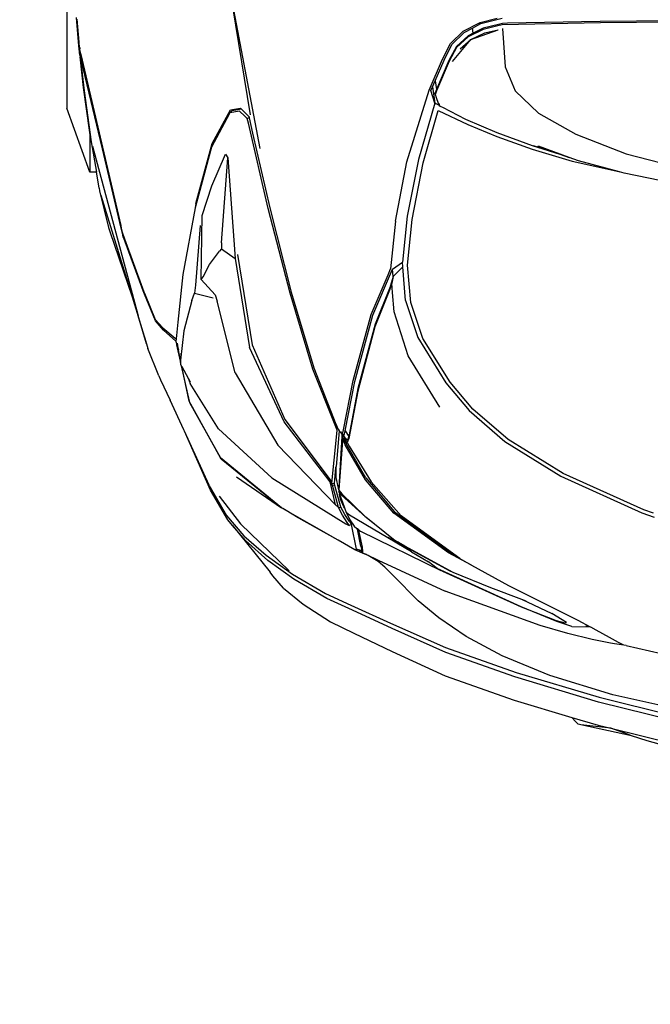
# Model space of a CAD drawing. Units: inches. Extents: x 22042254 to 25404563, y 17568978 to 17626777.
# Tile 21 of 45: x 22179809 to 22179830, y 17626194 to 17626227. Entities that reach past the tile are written whole.
import ezdxf

# ---------------------------------------------------------------- set-up
doc = ezdxf.new("R2010")
doc.units = ezdxf.units.IN
doc.header["$MEASUREMENT"] = 0
doc.layers.add('A-ANNO-DIMS', color=2, linetype='Continuous', lineweight=18)
doc.layers.add('A-SITE-VEHI', color=8, linetype='Continuous', lineweight=18)
doc.layers.add('Edges', color=250, linetype='Continuous')
doc.styles.get("Standard").update_dxf_attribs({"font": 'arial.ttf'})
doc.dimstyles.get("Standard").update_dxf_attribs({"dimtxt": 8, "dimasz": 0.18, "dimexe": 0.18, "dimexo": 0.0625, "dimgap": 0.09, "dimtad": 0, "dimtih": 1, "dimtoh": 1, "dimzin": 0, "dimdsep": 46, "dimlunit": 3, "dimtxsty": 'Standard', "dimcen": 0.09, "dimadec": 0, "dimazin": 0, "dimtfac": 1, "dimtofl": 0, "dimtmove": 0, "dimatfit": 3, "dimfxl": 1, "dimtolj": 1, "dimtzin": 0, "dimarcsym": 0})

# ---------------------------------------------------------------- blocks, each defined once
blk = doc.blocks.new('Nissan Qashqai pl')
at = {"layer": 'Edges'}
for p, q in [((11.05947, 11.55994), (11.06074, 11.45082)), ((11.06059, 11.56009), (11.06182, 11.4509)), ((11.6016, 11.52761), (11.58664, 11.46068)), ((11.58843, 11.44985), (11.60765, 11.5276)), ((11.61178, 11.52762), (11.59225, 11.44945)), ((11.61272, 11.45895), (11.62966, 11.52759)), ((11.16395, 11.47112), (11.17758, 11.52307)), ((11.18773, 11.51111), (11.17906, 11.46956)), ((11.54814, 11.47101), (11.55707, 11.51104)), ((11.62771, 11.50627), (11.62241, 11.48743)), ((11.44474, 11.49242), (11.44218, 11.48476)), ((11.44453, 11.48334), (11.44778, 11.49299)), ((11.44218, 11.48476), (11.41383, 11.42186)), ((11.41588, 11.41997), (11.44453, 11.48334)), ((11.62241, 11.48743), (11.61848, 11.47528)), ((11.61848, 11.47528), (11.61008, 11.43562)), ((11.61848, 11.47528), (11.61742, 11.47198)), ((11.14869, 11.43161), (11.16395, 11.47112)), ((11.17808, 11.46592), (11.1694, 11.43374)), ((11.17797, 11.4652), (11.17808, 11.46592)), ((11.17906, 11.46956), (11.17808, 11.46592)), ((11.54554, 11.46484), (11.54721, 11.46841)), ((11.54814, 11.47101), (11.54666, 11.46197)), ((11.61742, 11.47198), (11.61272, 11.45895)), ((11.1699, 11.42889), (11.17797, 11.4652)), ((11.53572, 11.44731), (11.54162, 11.45783)), ((11.54162, 11.45783), (11.54554, 11.46484)), ((11.54611, 11.45874), (11.54336, 11.44449)), ((11.54666, 11.46197), (11.54611, 11.45874)), ((11.58664, 11.46068), (11.57152, 11.41151)), ((11.61272, 11.45895), (11.61008, 11.43562)), ((11.61028, 11.44915), (11.61272, 11.45895)), ((11.06074, 11.45082), (11.06214, 11.37845)), ((11.06182, 11.4509), (11.06324, 11.37414)), ((11.52833, 11.43321), (11.53335, 11.4428)), ((11.53261, 11.43965), (11.5333, 11.44225)), ((11.53313, 11.42848), (11.53354, 11.44315)), ((11.5333, 11.44225), (11.53335, 11.4428)), ((11.53335, 11.4428), (11.53354, 11.44315)), ((11.53354, 11.44315), (11.53572, 11.44731)), ((11.54336, 11.44449), (11.53855, 11.42543)), ((11.56912, 11.38501), (11.58843, 11.44985)), ((11.59225, 11.44945), (11.57263, 11.38419)), ((11.60419, 11.42861), (11.61028, 11.44915)), ((11.61008, 11.43562), (11.60938, 11.43347)), ((11.1323, 11.40268), (11.14869, 11.43161)), ((11.16047, 11.39766), (11.1699, 11.42889)), ((11.1694, 11.43374), (11.1668, 11.42651)), ((11.5202, 11.41712), (11.52833, 11.43321)), ((11.53313, 11.42848), (11.52922, 11.417)), ((11.59084, 11.38361), (11.60419, 11.42861)), ((11.60772, 11.43162), (11.60419, 11.42861)), ((11.60938, 11.43347), (11.60772, 11.43162)), ((11.15764, 11.39828), (11.16426, 11.41918)), ((11.15766, 11.39771), (11.16426, 11.41918)), ((11.1668, 11.42651), (11.1582, 11.40259)), ((11.16426, 11.41918), (11.15826, 11.40186)), ((11.16426, 11.41918), (11.1668, 11.42651)), ((11.41383, 11.42186), (11.38718, 11.37878)), ((11.38877, 11.37638), (11.41588, 11.41997)), ((11.53009, 11.42439), (11.52299, 11.41307)), ((11.52855, 11.41625), (11.53022, 11.42324)), ((11.53022, 11.42324), (11.53009, 11.42439)), ((11.53855, 11.42543), (11.53253, 11.4038)), ((11.50131, 11.37908), (11.5202, 11.41712)), ((11.5118, 11.38938), (11.52299, 11.41307)), ((11.52922, 11.417), (11.51787, 11.38901)), ((11.51787, 11.38901), (11.52855, 11.41625)), ((11.57152, 11.41151), (11.55624, 11.37411)), ((11.53253, 11.4038), (11.50574, 11.32965)), ((11.11477, 11.38434), (11.1323, 11.40268)), ((11.14751, 11.37001), (11.15766, 11.39771)), ((11.15051, 11.36998), (11.16047, 11.39766)), ((11.51787, 11.38901), (11.48801, 11.32337)), ((11.49005, 11.3275), (11.51787, 11.38901)), ((11.50277, 11.36495), (11.5118, 11.38938)), ((11.5118, 11.38938), (11.51304, 11.39274)), ((11.09618, 11.37663), (11.11477, 11.38434)), ((11.54963, 11.33002), (11.56912, 11.38501)), ((11.57263, 11.38419), (11.5535, 11.33028)), ((11.57164, 11.32969), (11.59084, 11.38361)), ((11.06236, 11.3576), (11.05822, 11.37418)), ((11.06214, 11.37845), (11.06222, 11.37449)), ((11.06222, 11.37449), (11.06303, 11.37135)), ((11.06324, 11.37414), (11.06408, 11.37085)), ((11.06624, 11.37435), (11.09618, 11.37663)), ((11.38718, 11.37878), (11.3635, 11.35125)), ((11.36451, 11.34835), (11.38877, 11.37638)), ((11.48518, 11.35017), (11.50131, 11.37908)), ((11.55624, 11.37411), (11.54097, 11.34593)), ((11.06139, 11.35691), (11.05807, 11.37037)), ((11.06303, 11.37135), (11.06594, 11.3594)), ((11.06408, 11.37085), (11.06692, 11.35921)), ((11.06961, 11.36056), (11.0671, 11.37109)), ((11.07472, 11.34981), (11.0671, 11.37109)), ((11.13692, 11.34555), (11.14751, 11.37001)), ((11.14123, 11.34726), (11.15051, 11.36998)), ((11.06594, 11.3594), (11.06978, 11.35164)), ((11.06692, 11.35921), (11.0727, 11.34754)), ((11.07472, 11.34981), (11.06961, 11.36056)), ((11.49086, 11.33567), (11.50277, 11.36495)), ((11.06818, 11.34377), (11.06139, 11.35691)), ((11.06584, 11.35092), (11.06236, 11.3576)), ((11.06978, 11.35164), (11.06584, 11.35092)), ((11.06918, 11.34452), (11.06584, 11.35092)), ((11.06978, 11.35164), (11.07183, 11.3475)), ((11.3635, 11.35125), (11.34251, 11.3336)), ((11.48518, 11.35017), (11.4758, 11.33232)), ((11.48012, 11.34111), (11.48518, 11.35017)), ((11.07787, 11.3339), (11.06818, 11.34377)), ((11.07866, 11.33492), (11.06918, 11.34452)), ((11.07183, 11.3475), (11.08018, 11.33842)), ((11.0727, 11.34754), (11.0809, 11.33858)), ((11.08206, 11.34125), (11.07472, 11.34981)), ((11.092, 11.33548), (11.07472, 11.34981)), ((11.12767, 11.32749), (11.13692, 11.34555)), ((11.13017, 11.32416), (11.14123, 11.34726)), ((11.34283, 11.33026), (11.36451, 11.34835)), ((11.54097, 11.34593), (11.52646, 11.32473)), ((11.09081, 11.32882), (11.07866, 11.33492)), ((11.08018, 11.33842), (11.09121, 11.33249)), ((11.0809, 11.33858), (11.09174, 11.33271)), ((11.48005, 11.341), (11.44669, 11.29536)), ((11.47038, 11.29841), (11.49086, 11.33567)), ((11.47876, 11.33901), (11.47454, 11.33252)), ((11.47876, 11.33901), (11.48005, 11.341)), ((11.48005, 11.341), (11.48012, 11.34111)), ((11.48966, 11.33337), (11.49086, 11.33567)), ((11.09022, 11.32753), (11.07787, 11.3339)), ((11.11439, 11.31711), (11.09022, 11.32753)), ((11.10704, 11.32181), (11.09081, 11.32882)), ((11.09121, 11.33249), (11.1138, 11.3229)), ((11.09174, 11.33271), (11.11486, 11.323)), ((11.12645, 11.32495), (11.12767, 11.32749)), ((11.30757, 11.30833), (11.34283, 11.33026)), ((11.34251, 11.3336), (11.3082, 11.31215)), ((11.44331, 11.28988), (11.47454, 11.33252)), ((11.4758, 11.33232), (11.44474, 11.28965)), ((11.46332, 11.28473), (11.48966, 11.33337)), ((11.47038, 11.29841), (11.48966, 11.33337)), ((11.48133, 11.27727), (11.50574, 11.32965)), ((11.48983, 11.32694), (11.48954, 11.32636)), ((11.48983, 11.32694), (11.49005, 11.3275)), ((11.53062, 11.28691), (11.54963, 11.33002)), ((11.5535, 11.33028), (11.53487, 11.28826)), ((11.55274, 11.28821), (11.57164, 11.32969)), ((11.10704, 11.32181), (11.1138, 11.3229)), ((11.11164, 11.31982), (11.10704, 11.32181)), ((11.11164, 11.31982), (11.1244, 11.32146)), ((11.11467, 11.31851), (11.11164, 11.31982)), ((11.1138, 11.3229), (11.11393, 11.32284)), ((11.11393, 11.32284), (11.1164, 11.32172)), ((11.1244, 11.32146), (11.11467, 11.31851)), ((11.11486, 11.323), (11.1172, 11.32196)), ((11.1164, 11.32172), (11.1172, 11.32196)), ((11.11744, 11.32189), (11.1164, 11.32172)), ((11.1172, 11.32196), (11.11744, 11.32189)), ((11.11744, 11.32189), (11.11997, 11.32267)), ((11.11997, 11.32267), (11.12459, 11.32429)), ((11.12604, 11.32481), (11.1244, 11.32146)), ((11.1244, 11.32146), (11.12591, 11.32476)), ((11.1244, 11.32146), (11.16836, 11.30873)), ((11.12459, 11.32429), (11.12591, 11.32476)), ((11.12466, 11.32442), (11.12595, 11.32486)), ((11.12478, 11.32467), (11.12595, 11.32486)), ((11.12595, 11.32486), (11.1251, 11.3253)), ((11.12591, 11.32476), (11.12595, 11.32486)), ((11.12591, 11.32476), (11.12604, 11.32481)), ((11.12595, 11.32486), (11.12626, 11.32554)), ((11.12595, 11.32486), (11.12607, 11.32488)), ((11.12604, 11.32481), (11.12645, 11.32495)), ((11.12607, 11.32488), (11.12604, 11.32481)), ((11.12631, 11.32537), (11.12607, 11.32488)), ((11.12607, 11.32488), (11.12645, 11.32495)), ((11.17121, 11.31245), (11.13017, 11.32416)), ((11.36192, 11.32544), (11.32179, 11.30083)), ((11.45883, 11.26345), (11.48954, 11.32636)), ((11.48801, 11.32337), (11.48281, 11.31653)), ((11.52646, 11.32473), (11.51313, 11.30854)), ((11.17021, 11.29978), (11.11439, 11.31711)), ((11.21523, 11.3038), (11.17121, 11.31245)), ((11.3082, 11.31215), (11.28005, 11.30276)), ((11.47499, 11.30324), (11.48281, 11.31653)), ((11.16836, 11.30873), (11.21271, 11.29983)), ((11.2509, 11.3003), (11.21523, 11.3038)), ((11.27848, 11.29865), (11.30757, 11.30833)), ((11.51313, 11.30854), (11.49329, 11.28912)), ((11.21656, 11.2908), (11.17021, 11.29978)), ((11.21271, 11.29983), (11.24875, 11.29618)), ((11.25238, 11.29648), (11.24875, 11.29618)), ((11.2541, 11.28846), (11.24875, 11.29618)), ((11.28005, 11.30276), (11.2509, 11.3003)), ((11.27848, 11.29865), (11.25238, 11.29648)), ((11.25238, 11.29648), (11.25993, 11.28891)), ((11.32179, 11.30083), (11.28736, 11.28974)), ((11.47499, 11.30324), (11.4462, 11.25482)), ((11.46746, 11.29312), (11.47026, 11.29821)), ((11.47026, 11.29821), (11.47038, 11.29841)), ((11.21656, 11.2908), (11.25377, 11.28706)), ((11.25993, 11.28891), (11.2541, 11.28846)), ((11.29, 11.2731), (11.2541, 11.28846)), ((11.25993, 11.28891), (11.25999, 11.28889)), ((11.25999, 11.28889), (11.26503, 11.28789)), ((11.25999, 11.28889), (11.26771, 11.28668)), ((11.27242, 11.28847), (11.26503, 11.28789)), ((11.28736, 11.28974), (11.27242, 11.28847)), ((11.41708, 11.26758), (11.44331, 11.28988)), ((11.44474, 11.28965), (11.41866, 11.26734)), ((11.42028, 11.27173), (11.44669, 11.29536)), ((11.44691, 11.26684), (11.46587, 11.29022)), ((11.46538, 11.28932), (11.44788, 11.2676)), ((11.46538, 11.28932), (11.46587, 11.29022)), ((11.46587, 11.29022), (11.46737, 11.29293)), ((11.46746, 11.29312), (11.46737, 11.29293)), ((11.49329, 11.28912), (11.48692, 11.28262)), ((11.25857, 11.28503), (11.25377, 11.28706)), ((11.28951, 11.27177), (11.25857, 11.28503)), ((11.26503, 11.28789), (11.27055, 11.28622)), ((11.26771, 11.28668), (11.26785, 11.28663)), ((11.26785, 11.28663), (11.29721, 11.27493)), ((11.27055, 11.28622), (11.29928, 11.27468)), ((11.48692, 11.28262), (11.48256, 11.27724)), ((11.51652, 11.25601), (11.53062, 11.28691)), ((11.53487, 11.28826), (11.52058, 11.25724)), ((11.53843, 11.2583), (11.55274, 11.28821)), ((11.34188, 11.25916), (11.29, 11.2731)), ((11.29721, 11.27493), (11.34742, 11.26142)), ((11.29928, 11.27468), (11.34932, 11.2614)), ((11.47707, 11.26812), (11.48133, 11.27727)), ((11.48256, 11.27724), (11.47783, 11.26953)), ((11.48133, 11.27727), (11.48217, 11.27864)), ((11.3411, 11.25789), (11.28951, 11.27177)), ((11.41708, 11.26758), (11.38507, 11.24911)), ((11.41866, 11.26734), (11.3914, 11.25156)), ((11.39234, 11.25471), (11.42028, 11.27173)), ((11.42958, 11.2488), (11.44691, 11.26684)), ((11.44788, 11.2676), (11.43028, 11.24852)), ((11.47783, 11.26953), (11.47588, 11.26517)), ((11.47707, 11.26812), (11.47588, 11.26517)), ((11.37955, 11.25028), (11.3411, 11.25789)), ((11.38043, 11.25154), (11.34188, 11.25916)), ((11.34742, 11.26142), (11.38475, 11.2543)), ((11.34932, 11.2614), (11.38634, 11.25437)), ((11.44984, 11.25529), (11.45491, 11.25868)), ((11.47278, 11.2604), (11.45351, 11.25651)), ((11.45491, 11.25868), (11.45678, 11.26054)), ((11.4564, 11.26086), (11.45669, 11.26088)), ((11.45652, 11.26104), (11.45688, 11.26111)), ((11.45678, 11.26054), (11.45714, 11.2609)), ((11.45714, 11.2609), (11.45732, 11.2612)), ((11.45729, 11.26188), (11.45734, 11.2619)), ((11.47041, 11.26385), (11.45732, 11.2612)), ((11.45732, 11.2612), (11.45781, 11.262)), ((11.45736, 11.26195), (11.45734, 11.2619)), ((11.45736, 11.26195), (11.45755, 11.26195)), ((11.45781, 11.262), (11.45883, 11.26345)), ((11.45781, 11.262), (11.46047, 11.26254)), ((11.46047, 11.26254), (11.46049, 11.26254)), ((11.46049, 11.26254), (11.47129, 11.26473)), ((11.47322, 11.2592), (11.46579, 11.24614)), ((11.47041, 11.26385), (11.47423, 11.26446)), ((11.47129, 11.26473), (11.47442, 11.26498)), ((11.47269, 11.26007), (11.47281, 11.2603)), ((11.47463, 11.26457), (11.47278, 11.2604)), ((11.47423, 11.26446), (11.47278, 11.2604)), ((11.47278, 11.2604), (11.47281, 11.2603)), ((11.47281, 11.2603), (11.47317, 11.26096)), ((11.47281, 11.2603), (11.47322, 11.2592)), ((11.47585, 11.26509), (11.47322, 11.2592)), ((11.47423, 11.26446), (11.47445, 11.26449)), ((11.47442, 11.26498), (11.47433, 11.26475)), ((11.47442, 11.26498), (11.47446, 11.26498)), ((11.47445, 11.26477), (11.47446, 11.26498)), ((11.47463, 11.26457), (11.47445, 11.26449)), ((11.47446, 11.26498), (11.47482, 11.26501)), ((11.47585, 11.26509), (11.47463, 11.26457)), ((11.47482, 11.26501), (11.47475, 11.26484)), ((11.47482, 11.26501), (11.47585, 11.26509)), ((11.47588, 11.26517), (11.47585, 11.26509)), ((11.52949, 11.24004), (11.53843, 11.2583)), ((11.38338, 11.24949), (11.37955, 11.25028)), ((11.38043, 11.25154), (11.38475, 11.2543)), ((11.38408, 11.25081), (11.38043, 11.25154)), ((11.38295, 11.24897), (11.38801, 11.25321)), ((11.38408, 11.25081), (11.38338, 11.24949)), ((11.38475, 11.2543), (11.38801, 11.25321)), ((11.38823, 11.2519), (11.38491, 11.2491)), ((11.38811, 11.25194), (11.3861, 11.25078)), ((11.38634, 11.25437), (11.38953, 11.25299)), ((11.3914, 11.25156), (11.3867, 11.24922)), ((11.38862, 11.25223), (11.38822, 11.252)), ((11.38862, 11.25223), (11.38823, 11.2519)), ((11.39063, 11.25338), (11.38862, 11.25223)), ((11.38953, 11.25299), (11.38862, 11.25223)), ((11.38953, 11.25299), (11.39234, 11.25471)), ((11.41698, 11.19425), (11.45295, 11.25195)), ((11.4397, 11.25049), (11.43368, 11.248)), ((11.43609, 11.24937), (11.44061, 11.25095)), ((11.44061, 11.25095), (11.4397, 11.25049)), ((11.44573, 11.25131), (11.43996, 11.24823)), ((11.44061, 11.25095), (11.44418, 11.2522)), ((11.44418, 11.2522), (11.44968, 11.25519)), ((11.4462, 11.25482), (11.44418, 11.2522)), ((11.45121, 11.25489), (11.44573, 11.25131)), ((11.45199, 11.25317), (11.44624, 11.24948)), ((11.44968, 11.25519), (11.44984, 11.25529)), ((11.44984, 11.25529), (11.45351, 11.25651)), ((11.45121, 11.25489), (11.45351, 11.25651)), ((11.45386, 11.25448), (11.45199, 11.25317)), ((11.45295, 11.25195), (11.45421, 11.25473)), ((11.45316, 11.25595), (11.45351, 11.25651)), ((11.45351, 11.25651), (11.45421, 11.25473)), ((11.45421, 11.25473), (11.45386, 11.25448)), ((11.47197, 11.25711), (11.47177, 11.25676)), ((11.50736, 11.23616), (11.51652, 11.25601)), ((11.52058, 11.25724), (11.51126, 11.23721)), ((11.33108, 11.22699), (11.37506, 11.24429)), ((11.37475, 11.24309), (11.33228, 11.22637)), ((11.38, 11.24532), (11.37475, 11.24309)), ((11.37506, 11.24429), (11.37524, 11.24436)), ((11.37506, 11.24429), (11.37621, 11.24429)), ((11.37922, 11.24593), (11.37524, 11.24436)), ((11.3763, 11.24436), (11.37524, 11.24436)), ((11.37922, 11.24593), (11.38041, 11.24692)), ((11.37933, 11.24631), (11.37922, 11.24593)), ((11.38533, 11.24487), (11.38, 11.24532)), ((11.38041, 11.24692), (11.38275, 11.24887)), ((11.38041, 11.24692), (11.40818, 11.24436)), ((11.38129, 11.24847), (11.38167, 11.2488)), ((11.38275, 11.24887), (11.38338, 11.24949)), ((11.38446, 11.24984), (11.38295, 11.24897)), ((11.38295, 11.24897), (11.38491, 11.2491)), ((11.38295, 11.24897), (11.38461, 11.24885)), ((11.38461, 11.24885), (11.38464, 11.24887)), ((11.38461, 11.24885), (11.38934, 11.2486)), ((11.38464, 11.24887), (11.38501, 11.24911)), ((11.38491, 11.2491), (11.38464, 11.24887)), ((11.38501, 11.24911), (11.38507, 11.24911)), ((11.38507, 11.24911), (11.3867, 11.24922)), ((11.42115, 11.24117), (11.38533, 11.24487)), ((11.3867, 11.24922), (11.3915, 11.24906)), ((11.38934, 11.2486), (11.42481, 11.24653)), ((11.3915, 11.24906), (11.42659, 11.2465)), ((11.3915, 11.19885), (11.4381, 11.24397)), ((11.41644, 11.24436), (11.40818, 11.24436)), ((11.40898, 11.24429), (11.40818, 11.24436)), ((11.40898, 11.24429), (11.4163, 11.24429)), ((11.4152, 11.24371), (11.40898, 11.24429)), ((11.4163, 11.24429), (11.4152, 11.24371)), ((11.42154, 11.24313), (11.4152, 11.24371)), ((11.41644, 11.24436), (11.4163, 11.24429)), ((11.41686, 11.24458), (11.41644, 11.24436)), ((11.4252, 11.2462), (11.41686, 11.24458)), ((11.42115, 11.24117), (11.42154, 11.24313)), ((11.42296, 11.24352), (11.42154, 11.24313)), ((11.43154, 11.24397), (11.42287, 11.24164)), ((11.42296, 11.24352), (11.42287, 11.24164)), ((11.43996, 11.24823), (11.42296, 11.24352)), ((11.42481, 11.24653), (11.42659, 11.2465)), ((11.42659, 11.2465), (11.4252, 11.2462)), ((11.42659, 11.2465), (11.42684, 11.24649)), ((11.42684, 11.24649), (11.42958, 11.2488)), ((11.42684, 11.24649), (11.42784, 11.24647)), ((11.43028, 11.24852), (11.42784, 11.24647)), ((11.42784, 11.24647), (11.42996, 11.24721)), ((11.4381, 11.24397), (11.42915, 11.24177)), ((11.42996, 11.24721), (11.43609, 11.24937)), ((11.43368, 11.248), (11.42996, 11.24721)), ((11.44027, 11.24637), (11.43154, 11.24397)), ((11.4381, 11.24397), (11.44027, 11.24637)), ((11.44027, 11.24637), (11.43996, 11.24823)), ((11.44624, 11.24948), (11.44027, 11.24637)), ((11.44114, 11.20281), (11.46562, 11.24583)), ((11.44697, 11.21272), (11.46562, 11.24583)), ((11.46562, 11.24583), (11.46579, 11.24614)), ((11.3715, 11.20434), (11.41772, 11.23895)), ((11.42033, 11.23975), (11.37334, 11.20375)), ((11.41772, 11.23895), (11.41931, 11.23998)), ((11.41915, 11.23969), (11.4194, 11.23996)), ((11.41931, 11.23998), (11.4196, 11.24017)), ((11.4194, 11.23996), (11.41931, 11.23998)), ((11.4194, 11.23996), (11.4196, 11.24017)), ((11.41958, 11.23992), (11.4194, 11.23996)), ((11.4196, 11.24017), (11.42014, 11.24052)), ((11.41984, 11.24006), (11.42014, 11.24052)), ((11.42014, 11.24052), (11.42115, 11.24117)), ((11.42915, 11.24177), (11.42033, 11.23975)), ((11.42287, 11.24164), (11.42033, 11.23975)), ((11.42178, 11.24134), (11.42115, 11.24117)), ((11.42287, 11.24164), (11.42178, 11.24134)), ((11.42216, 11.24127), (11.42178, 11.24134)), ((11.49236, 11.21027), (11.50736, 11.23616)), ((11.51126, 11.23721), (11.49628, 11.21137)), ((11.51576, 11.21859), (11.52949, 11.24004)), ((11.27199, 11.20923), (11.33108, 11.22699)), ((11.33228, 11.22637), (11.27276, 11.20843)), ((11.44697, 11.21272), (11.44114, 11.20281)), ((11.50327, 11.20341), (11.51576, 11.21859)), ((11.20627, 11.19262), (11.27199, 11.20923)), ((11.27276, 11.20843), (11.20665, 11.19145)), ((11.31316, 11.17892), (11.3715, 11.20434)), ((11.45306, 11.16974), (11.48975, 11.20767)), ((11.47745, 11.18983), (11.49236, 11.21027)), ((11.49628, 11.21137), (11.48154, 11.19102)), ((11.37334, 11.20375), (11.31527, 11.17691)), ((11.33497, 11.16556), (11.3915, 11.19885)), ((11.44046, 11.20182), (11.40144, 11.15414)), ((11.40216, 11.15476), (11.44046, 11.20182)), ((11.41633, 11.16662), (11.44046, 11.20182)), ((11.44081, 11.20225), (11.44046, 11.20182)), ((11.4411, 11.20277), (11.44081, 11.20225)), ((11.44114, 11.20281), (11.4411, 11.20277)), ((11.50327, 11.20341), (11.49363, 11.19502)), ((11.20665, 11.19145), (11.14012, 11.17593)), ((11.14803, 11.17913), (11.20627, 11.19262)), ((11.37896, 11.15265), (11.41698, 11.19425)), ((11.45433, 11.16358), (11.49082, 11.19282)), ((11.46237, 11.17248), (11.47745, 11.18983)), ((11.48154, 11.19102), (11.46617, 11.17358)), ((11.49363, 11.19502), (11.49082, 11.19282)), ((11.03575, 11.16129), (11.1598, 11.18473)), ((11.04919, 11.16347), (11.13359, 11.17719)), ((11.12929, 11.17052), (11.13526, 11.17642)), ((11.1347, 11.17313), (11.13062, 11.16899)), ((11.13658, 11.17502), (11.1347, 11.17313)), ((11.13526, 11.17642), (11.13585, 11.17654)), ((11.13585, 11.17654), (11.14803, 11.17913)), ((11.13585, 11.17654), (11.13658, 11.17502)), ((11.14012, 11.17593), (11.13658, 11.17502)), ((11.24278, 11.16729), (11.31316, 11.17892)), ((11.24587, 11.16563), (11.31527, 11.17691)), ((11.46617, 11.17358), (11.45433, 11.16358)), ((11.12846, 11.16971), (11.12929, 11.17052)), ((11.12977, 11.16183), (11.12846, 11.16971)), ((11.12929, 11.17052), (11.13057, 11.16299)), ((11.13062, 11.16899), (11.13192, 11.16144)), ((11.16717, 11.15976), (11.24587, 11.16563)), ((11.23823, 11.15494), (11.24587, 11.16563)), ((11.33497, 11.16556), (11.27913, 11.15147)), ((11.43143, 11.15309), (11.45306, 11.16974)), ((11.44642, 11.15882), (11.46237, 11.17248)), ((11.15597, 11.14759), (11.12977, 11.16183)), ((11.13192, 11.16144), (11.13057, 11.16299)), ((11.13192, 11.16144), (11.13652, 11.15905)), ((11.13652, 11.15905), (11.15893, 11.14704)), ((11.16444, 11.15792), (11.16717, 11.15976)), ((11.18896, 11.14734), (11.16444, 11.15792)), ((11.23369, 11.15498), (11.16717, 11.15976)), ((11.42433, 11.14593), (11.44642, 11.15882)), ((11.44983, 11.15977), (11.42671, 11.14629)), ((11.45433, 11.16358), (11.44983, 11.15977)), ((11.23369, 11.15498), (11.23823, 11.15494)), ((11.23823, 11.15494), (11.2401, 11.15337)), ((11.25046, 11.1455), (11.2401, 11.15337)), ((11.27429, 11.14993), (11.27913, 11.15147)), ((11.37896, 11.15265), (11.34336, 11.13032)), ((11.40144, 11.15414), (11.3571, 11.12956)), ((11.35832, 11.12998), (11.40144, 11.15414)), ((11.40216, 11.15476), (11.40144, 11.15414)), ((11.20291, 11.13489), (11.15597, 11.14759)), ((11.15893, 11.14704), (11.20616, 11.13437)), ((11.2121, 11.1399), (11.18896, 11.14734)), ((11.26005, 11.1405), (11.25046, 11.1455)), ((11.27429, 11.14993), (11.26224, 11.13901)), ((11.27289, 11.13379), (11.27664, 11.14845)), ((11.42671, 11.14629), (11.38067, 11.12595)), ((11.42283, 11.14525), (11.38067, 11.12595)), ((11.42283, 11.14525), (11.42433, 11.14593)), ((11.20291, 11.13489), (11.20295, 11.13488)), ((11.20295, 11.13488), (11.20616, 11.13437)), ((11.26224, 11.13901), (11.2121, 11.1399)), ((11.21991, 11.1382), (11.26663, 11.13449)), ((11.26224, 11.13901), (11.26005, 11.1405)), ((11.20616, 11.13437), (11.25827, 11.12461)), ((11.26663, 11.13449), (11.27289, 11.13379)), ((11.27871, 11.13184), (11.27289, 11.13379)), ((11.27871, 11.13184), (11.30218, 11.1256)), ((11.32955, 11.12347), (11.3571, 11.12956)), ((11.3571, 11.12956), (11.33021, 11.12384)), ((11.33021, 11.12384), (11.33938, 11.12898)), ((11.33938, 11.12898), (11.34202, 11.13045)), ((11.33938, 11.12898), (11.34336, 11.13032)), ((11.3571, 11.12956), (11.35832, 11.12998)), ((11.25827, 11.12461), (11.29558, 11.12077)), ((11.29558, 11.12077), (11.30849, 11.1195)), ((11.30218, 11.1256), (11.32517, 11.12286)), ((11.30805, 11.11884), (11.30863, 11.11948)), ((11.30813, 11.11883), (11.30863, 11.11948)), ((11.30849, 11.1195), (11.30863, 11.11948)), ((11.30863, 11.11948), (11.31033, 11.1193)), ((11.31033, 11.1193), (11.31027, 11.11923)), ((11.31033, 11.1193), (11.31061, 11.11927)), ((11.31061, 11.11927), (11.314, 11.12039)), ((11.31704, 11.12142), (11.31186, 11.12058)), ((11.31323, 11.11986), (11.32588, 11.12266)), ((11.32423, 11.12258), (11.314, 11.12039)), ((11.314, 11.12039), (11.31704, 11.12142)), ((11.32423, 11.12258), (11.31704, 11.12142)), ((11.31982, 11.1231), (11.32517, 11.12286)), ((11.32423, 11.12258), (11.32588, 11.12266)), ((11.32517, 11.12286), (11.32831, 11.12278)), ((11.32588, 11.12266), (11.32831, 11.12278)), ((11.32831, 11.12278), (11.32955, 11.12347)), ((11.32955, 11.12347), (11.33021, 11.12384)), ((11.37962, 11.12547), (11.35656, 11.11477)), ((11.38067, 11.12595), (11.37962, 11.12547)), ((11.30003, 11.10916), (11.30813, 11.11883)), ((11.31027, 11.11923), (11.30178, 11.10961)), ((11.34052, 11.10725), (11.35656, 11.11477)), ((11.29339, 11.10313), (11.30003, 11.10916)), ((11.30178, 11.10961), (11.29459, 11.10327)), ((11.33757, 11.10603), (11.31612, 11.09747)), ((11.33757, 11.10603), (11.34052, 11.10725)), ((11.29459, 11.10327), (11.27358, 11.0947)), ((11.27407, 11.09522), (11.29339, 11.10313)), ((11.27568, 11.08503), (11.31244, 11.09628)), ((11.31244, 11.09628), (11.29065, 11.08989)), ((11.31244, 11.09628), (11.31612, 11.09747)), ((11.15816, 11.05423), (11.29065, 11.08989)), ((11.2732, 11.09452), (11.22772, 11.07792)), ((11.23038, 11.07923), (11.27187, 11.09432)), ((11.27187, 11.09432), (11.27407, 11.09522)), ((11.27358, 11.0947), (11.2732, 11.09452)), ((11.27358, 11.0947), (11.27407, 11.09522)), ((11.30801, 11.09508), (11.30877, 11.09528)), ((11.19633, 11.06072), (11.27568, 11.08503)), ((11.22475, 11.06772), (11.27568, 11.08503)), ((11.08649, 11.04496), (11.21998, 11.07614)), ((11.22216, 11.0766), (11.08821, 11.045)), ((11.09177, 11.04531), (11.22216, 11.0766)), ((11.21998, 11.07614), (11.22216, 11.0766)), ((11.2222, 11.07656), (11.22216, 11.0766)), ((11.22715, 11.07771), (11.2222, 11.07656)), ((11.22238, 11.07665), (11.2222, 11.07656)), ((11.22238, 11.07665), (11.22532, 11.07737)), ((11.22532, 11.07737), (11.23038, 11.07923)), ((11.22731, 11.07783), (11.22706, 11.07777)), ((11.22962, 11.07837), (11.22715, 11.07771)), ((11.22772, 11.07792), (11.22715, 11.07771)), ((11.22962, 11.07837), (11.22772, 11.07792)), ((11.19297, 11.05964), (11.22148, 11.06662)), ((11.22148, 11.06662), (11.22475, 11.06772)), ((11.19065, 11.05923), (11.17828, 11.05716)), ((11.19089, 11.05929), (11.19065, 11.05923)), ((11.19089, 11.05929), (11.19297, 11.05964)), ((11.14751, 11.05208), (11.11234, 11.04716)), ((11.11474, 11.04762), (11.15472, 11.05317)), ((11.17828, 11.05208), (11.12828, 11.03408)), ((11.15248, 11.05278), (11.14751, 11.05208)), ((11.14751, 11.05208), (11.17828, 11.05208)), ((11.15472, 11.05317), (11.15248, 11.05278)), ((11.15472, 11.05317), (11.17828, 11.05716)), ((11.17828, 11.05716), (11.17828, 11.05208)), ((11.07977, 11.04339), (11.05762, 11.04159)), ((11.05899, 11.04188), (11.07681, 11.04337)), ((11.07681, 11.04337), (11.08106, 11.04371)), ((11.08696, 11.04422), (11.07977, 11.04339)), ((11.08106, 11.04371), (11.08273, 11.0441)), ((11.08114, 11.04436), (11.08208, 11.0442)), ((11.08273, 11.0441), (11.08562, 11.04476)), ((11.08273, 11.0441), (11.08365, 11.04395)), ((11.08821, 11.045), (11.08365, 11.04395)), ((11.08365, 11.04395), (11.08696, 11.04422)), ((11.08562, 11.04476), (11.08649, 11.04496)), ((11.08649, 11.04496), (11.08796, 11.04514)), ((11.08696, 11.04422), (11.08721, 11.04424)), ((11.08728, 11.04426), (11.08721, 11.04424)), ((11.08728, 11.04426), (11.08834, 11.04438)), ((11.08834, 11.04438), (11.11474, 11.04762)), ((11.11234, 11.04716), (11.08834, 11.04438)), ((10.95773, 11.03408), (11.12828, 11.03408))]:
    blk.add_line(p, q, dxfattribs=at)
blk = doc.blocks.new('CAR')
blk.add_blockref('Nissan Qashqai pl', (-9.74328, -11.91512))
blk = doc.blocks.new('*D59')
at = {"layer": 'A-ANNO-DIMS', "color": 0, "lineweight": -2, "transparency": 16777216}
for p, q in [((22179802.402, 17626200.497), (22179802.402, 17626171.756)), ((22179895.926, 17626200.497), (22179895.926, 17626171.756)), ((22179802.582, 17626171.936), (22179829.153, 17626171.936)), ((22179895.746, 17626171.936), (22179869.175, 17626171.936))]:
    blk.add_line(p, q, dxfattribs=at)
at = {"layer": 'A-ANNO-DIMS', "color": 0, "transparency": 16777216}
for points in [[(22179802.582, 17626171.966), (22179802.582, 17626171.906), (22179802.402, 17626171.936)], [(22179895.746, 17626171.966), (22179895.746, 17626171.906), (22179895.926, 17626171.936)]]:
    blk.add_solid(points, dxfattribs=at)
at = {"layer": 'Defpoints', "color": 0, "transparency": 16777216}
for p in [(22179802.402, 17626200.559), (22179895.926, 17626200.559), (22179895.926, 17626171.936)]:
    blk.add_point(p, dxfattribs=at)
at = {"layer": 'A-ANNO-DIMS', "color": 0, "transparency": 16777216, "insert": (22179849.164, 17626171.936), "char_height": 8, "attachment_point": 5}
blk.add_mtext('\\A1;7\'-9 1/2"', dxfattribs=at)

msp = doc.modelspace()

# ---------------------------------------------------------------- block references
at = {"layer": 'A-SITE-VEHI', "xscale": 43.56002006885659, "yscale": 43.56002006885659, "zscale": 43.56002006885659, "rotation": 270}
msp.add_blockref('CAR', (22179848.861, 17626284.325), dxfattribs=at)

# ---------------------------------------------------------------- dimensions: what is measured, and where the dimension line sits
at = {"layer": 'A-ANNO-DIMS'}
dim = msp.add_linear_dim(base=(22179895.926, 17626171.936), p1=(22179802.402, 17626200.559), p2=(22179895.926, 17626200.559), dimstyle='Standard', override={"dimdec": 1, "dimlfac": 1, "dimrnd": 0, "dimzin": 1, "dimdsep": 46, "dimlunit": 4, "dimfrac": 2}, dxfattribs=at)
dim.commit()
dim.dimension.update_dxf_attribs({"geometry": '*D59', "text_midpoint": (22179849.164, 17626171.936)})

doc.saveas('drawing.dxf')
